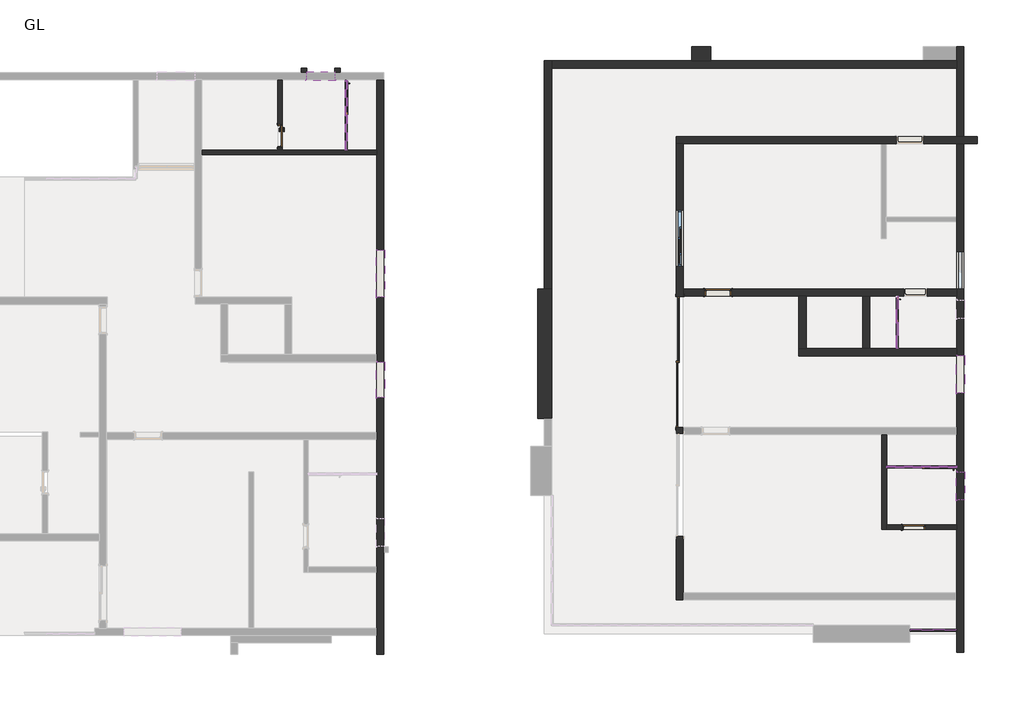
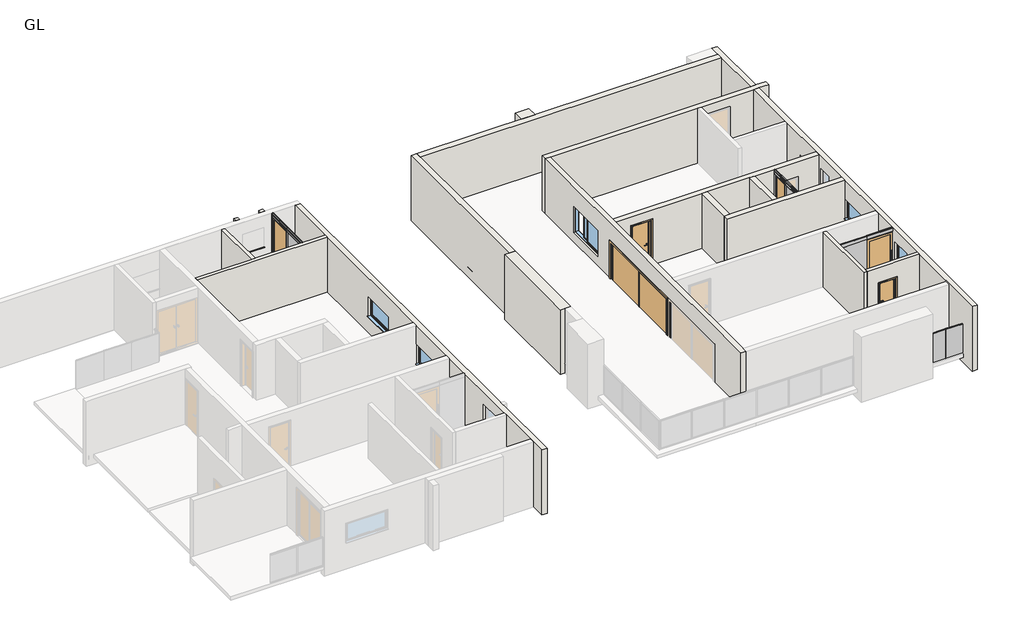
# One storey, part 4 of 6: 41 members, 18 walls, 11 plates, 7 doors, 6 windows.
# Revit data of these elements (continued)
# Type "Windows_Sgl_Plain : 3'10\"" (continued)
#   Vis - Cavity Closers = yes
#   Define Thermal Properties by = 1
#   Material Trim = Window Frame
#   Material Glass = Glass
#   Material Frame = Window Frame
#   Wall Closure = (empty or 0)
# Type "Windows_Sgl_Plain : 4'"
#   Type Mark = "65"
#   Operation = "SinglePanel"
#   Construction Type Id = "SGL"
#   Manufacturer = "Revit"
#   Keynote = "L10"
#   Analytic Construction = "Large single-glazed windows"
#   Wrap Layers (Ext) from Ext = 0' - 4.03543"
#   Wrap Layers (Int) from Ext = 0' - 6.98819"
#   Window Board Projection = 0' - 0.98425"
#   Window Board Extension = 0' - 0.98425"
#   Visual Light Transmittance = 0.9
#   Solar Heat Gain Coefficient = 0.86
#   Rough Width = 4' - 0"
#   Rough Height = 2' - 11.82677"
#   Height = 2' - 11.82677"
#   Width = 4' - 0"
#   Heat Transfer Coefficient (U) = 5.5617 W/(m²·K)
#   Glazing Thickness = 0' - 0.94488"
#   FrameOffset - External = 0' - 1.9685"
#   Frame Depth = 0' - 2.55906"
#   Default Head Height = 6' - 11.07087"
#   Cill Depth = 0' - 3.44488"
#   Cavity Closer Width = 0' - 1.9685"
#   Cavity Closer Offset from Ext = 0' - 4.03543"
#   Cavity Closer Depth = 0' - 3.34646"
#   Vis - Cavity Closers = yes
#   Define Thermal Properties by = 1
#   Material Trim = Window Frame
#   Material Glass = Glass
#   Material Frame = Window Frame
#   Wall Closure = (empty or 0)
# Type "Windows_Sgl_Plain : 5'"
#   Type Mark = "67"
#   Operation = "SinglePanel"
#   Construction Type Id = "SGL"
#   Manufacturer = "Revit"
#   Keynote = "L10"
#   Analytic Construction = "Large single-glazed windows"
#   Wrap Layers (Ext) from Ext = 0' - 4.03543"
#   Wrap Layers (Int) from Ext = 0' - 6.98819"
#   Window Board Projection = 0' - 0.98425"
#   Window Board Extension = 0' - 0.98425"
#   Visual Light Transmittance = 0.9
#   Solar Heat Gain Coefficient = 0.86
#   Rough Width = 5' - 0"
#   Rough Height = 2' - 11.82677"
#   Height = 2' - 11.82677"
#   Width = 5' - 0"
#   Heat Transfer Coefficient (U) = 5.5617 W/(m²·K)
#   Glazing Thickness = 0' - 0.94488"
#   FrameOffset - External = 0' - 1.9685"
#   Frame Depth = 0' - 2.55906"
#   Default Head Height = 6' - 11.07087"
#   Cill Depth = 0' - 3.44488"
#   Cavity Closer Width = 0' - 1.9685"
#   Cavity Closer Offset from Ext = 0' - 4.03543"
#   Cavity Closer Depth = 0' - 3.34646"
#   Vis - Cavity Closers = yes
#   Define Thermal Properties by = 1
#   Material Trim = Window Frame
#   Material Glass = Glass
#   Material Frame = Window Frame
#   Wall Closure = (empty or 0)
# Element 1 (IfcDoor, "14'")
#   Phase Created = New Construction
#   Materials on its faces: "Puerta - Panel", "Cristal"
# Element 2 (IfcDoor, "Doors_IntSgl : 2'11\"")
#   Phase Created = New Construction
#   Materials on its faces: "Door - Architrave", "Door - Handle", "Door - Frame/Mullion (1)", "Door - Panel"
# Elements 3, 4 (IfcDoor, "Doors_IntSgl : 2.5'")
#   Phase Created = New Construction
#   Materials on its faces: "Door - Architrave", "Door - Handle", "Door - Frame/Mullion (1)", "Door - Panel"
# Elements 5, 6, 7 (IfcDoor, "Doors_Sgl_Glass_1 : Glass_Panel-12mm_Thickness")
#   Phase Created = New Construction
#   Materials on its faces: "Metal - Aluminum", "Glass"
# Elements 8, 9, 10, 11, 12, 13, 14, 15, 16, 17, 18, 19, 20, 21, 22, 23, 24, 25, 26, 27, 28, 29, 30, 31, 32, 33, 34, 35, 36, 37, 38, 39, 40, 41, 42, 43, 44, 45, 46, 47, 48 (IfcMember, "Rectangular Mullion : 30mm_Square")
#   Phase Created = New Construction
#   Materials on its faces: "Aluminium"
# Elements 49, 50, 51, 52, 53, 54, 55, 56, 57, 58, 59 (IfcPlate, "System Panel : Glazed")
#   Phase Created = New Construction
#   Materials on its faces: "Glass"
# Elements 60, 61 (IfcWall, "1'6\"")
#   Top Offset = 0' - 0"
#   Base Offset = 0' - 0"
#   wall height = 9' - 10.11024"
#   Phase Created = New Construction
#   Base Constraint = GL
#   Top Constraint = FFL
#   Materials on its faces: "Brick, Common"
# Elements 62, 63 (IfcWall, "10\"")
#   Top Offset = 0' - 0"
#   Base Offset = 0' - 0"
#   wall height = 9' - 10.11024"
#   Phase Created = New Construction
#   Base Constraint = GL
#   Top Constraint = FFL
#   Materials on its faces: "Brick, Common"
# Elements 64, 65, 66, 67 (IfcWall, "6\" WALL")
#   Top Offset = 0' - 0"
#   Base Offset = 0' - 0"
#   wall height = 9' - 10.11024"
#   Phase Created = New Construction
#   Base Constraint = GL
#   Top Constraint = FFL
#   Materials on its faces: "Brick, Common"
# Elements 68, 69 (IfcWall, "7\" WALL")
#   Top Offset = 0' - 0"
#   Base Offset = 0' - 0"
#   wall height = 9' - 10.11024"
#   Phase Created = New Construction
#   Base Constraint = GL
#   Top Constraint = FFL
#   Materials on its faces: "Brick, Common"
# Elements 70, 71, 72, 73, 74, 75, 76, 77 (IfcWall, "9\" INNER WALL")
#   Top Offset = 0' - 0"
#   Base Offset = 0' - 0"
#   wall height = 9' - 10.11024"
#   Phase Created = New Construction
#   Base Constraint = GL
#   Top Constraint = FFL
#   Materials on its faces: "Brick, Common"
# Element 78 (IfcWindow, "Parametric_Operable_Sliding_Window_6387 : 6'")
#   Mark = "5"
#   Opened Pane Portion = 1' - 7.68504"
#   Phase Created = New Construction
#   Materials on its faces: "Window Frame", "Window Glass"
# Element 79 (IfcWindow, "Windows_Sgl_Plain : 3'")
#   Mark = "10"
#   Phase Created = New Construction
#   Materials on its faces: "Window Frame", "Glass"
# Element 80 (IfcWindow, "Windows_Sgl_Plain : 3'")
#   Mark = "12"
#   Phase Created = New Construction
#   Materials on its faces: "Window Frame", "Glass"
# Element 81 (IfcWindow, "Windows_Sgl_Plain : 3'10\"")
#   Mark = "14"
#   Phase Created = New Construction
#   Materials on its faces: "Window Frame", "Glass"
# Element 82 (IfcWindow, "Windows_Sgl_Plain : 4'")
#   Mark = "9"
#   Phase Created = New Construction
#   Materials on its faces: "Window Frame", "Glass"
# Element 83 (IfcWindow, "Windows_Sgl_Plain : 5'")
#   Mark = "13"
#   Phase Created = New Construction
#   Materials on its faces: "Window Frame", "Glass"
# Materials
#   "Puerta - Panel": class "Madera", colour RGB 210 159 95, transparency 0
#   "Door - Handle": colour RGB 0 0 0, transparency 0, Keynote = "P21", Cost = 0
#   "Door - Frame/Mullion (1)": class "Wood", colour RGB 212 179 113, transparency 0, Keynote = "L20", Cost = 0
#   "Door - Panel": class "Wood", colour RGB 210 159 95, transparency 0, Keynote = "L20", Cost = 0
#   "Door - Architrave": class "Wood", colour RGB 154 90 5, transparency 0, Keynote = "P20", Cost = 0
#   "Metal - Aluminum": class "Metal", colour RGB 247 247 247, transparency 0
#   "Glass": class "Glass", colour RGB 0 128 192, transparency 0.9, Description = "Soda Lime Glass", Cost = 0
#   "Brick, Common": class "Masonry", colour RGB 170 100 105, transparency 0, Description = "Common brick", Cost = 0
#   "Window Reveal": colour RGB 255 255 255, transparency 0
#   "Window Glass": colour RGB 0 0 255, transparency 0.75
#   "Window Frame": colour RGB 249 249 249, transparency 0, Keynote = "L10", Cost = 0
#   "Window Architrave": colour RGB 255 255 255, transparency 0
#   "Cristal": class "Vidrio", colour RGB 0 0 255, transparency 0.75
#   "Aluminium": class "Metal", colour RGB 247 247 247, transparency 0, Description = "Aluminium 6061", Cost = 0
